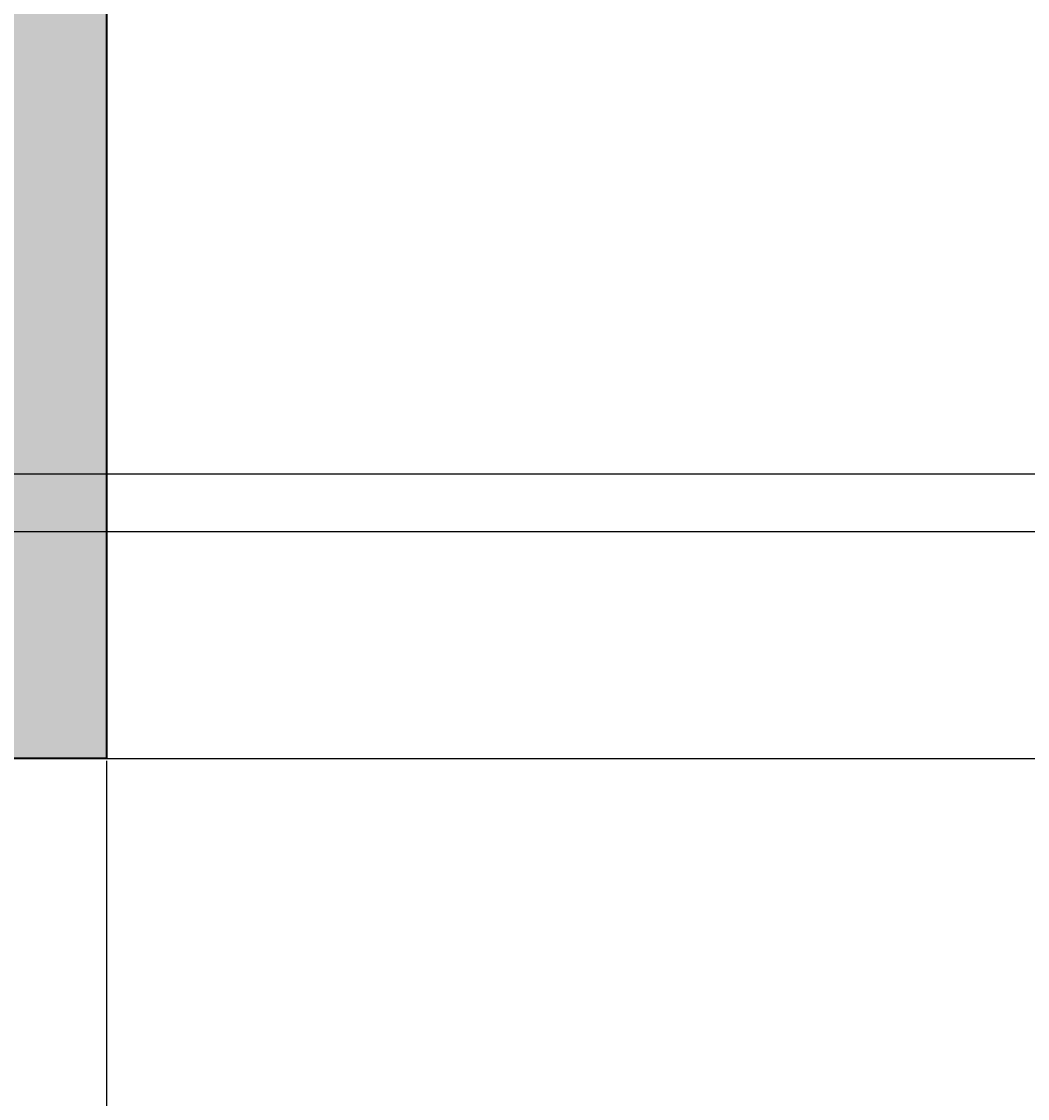
# Model space of a CAD drawing. Units: inches. Extents: x 1998 to 2588, y 1139 to 1977.
# Tile 95 of 134: x 2344 to 2370, y 1580 to 1608. Entities that reach past the tile are written whole.
import ezdxf

# ---------------------------------------------------------------- set-up
doc = ezdxf.new("R2010")
doc.units = ezdxf.units.IN
for name, color, linetype, lineweight in [('A-ANNO-DIMS', 2, 'Continuous', 18), ('A-WALL-PATT', 252, 'Continuous', 13), ('WALL', 200, 'Continuous', 35)]:
    doc.layers.add(name, color=color, linetype=linetype, lineweight=lineweight)
doc.styles.get("Standard").update_dxf_attribs({"font": 'arial.ttf'})
doc.dimstyles.get("Standard").update_dxf_attribs({"dimtxt": 0.18, "dimasz": 0.18, "dimexe": 0.18, "dimexo": 0.0625, "dimgap": 0.09, "dimtad": 0, "dimtih": 1, "dimtoh": 1, "dimdec": 4, "dimzin": 0, "dimdsep": 46, "dimtxsty": 'Standard', "dimcen": 0.09, "dimadec": 0, "dimazin": 0, "dimtfac": 1, "dimtdec": 4, "dimtofl": 0, "dimtmove": 0, "dimatfit": 3, "dimfxl": 1, "dimtolj": 1, "dimtzin": 0, "dimarcsym": 0})

# ---------------------------------------------------------------- blocks, each defined once
blk = doc.blocks.new('*D30')
at = {"layer": 'A-ANNO-DIMS', "color": 0, "lineweight": -2, "transparency": 16777216}
for p, q in [((2407.91, 1636.732), (1997.843, 1636.732)), ((1998.023, 1636.552), (1998.023, 1615.913)), ((1998.023, 1594.912), (1998.023, 1615.552)), ((2407.91, 1594.732), (1997.843, 1594.732))]:
    blk.add_line(p, q, dxfattribs=at)
at = {"layer": 'A-ANNO-DIMS', "color": 0, "transparency": 16777216}
for points in [[(1997.993, 1636.552), (1998.053, 1636.552), (1998.023, 1636.732)], [(1997.993, 1594.912), (1998.053, 1594.912), (1998.023, 1594.732)]]:
    blk.add_solid(points, dxfattribs=at)
at = {"layer": 'Defpoints', "color": 0, "transparency": 16777216}
for p in [(1998.023, 1636.732), (2407.973, 1636.732), (2407.973, 1594.732)]:
    blk.add_point(p, dxfattribs=at)
at = {"layer": 'A-ANNO-DIMS', "color": 0, "transparency": 16777216, "insert": (1998.023, 1615.732), "char_height": 0.18, "attachment_point": 5}
blk.add_mtext('\\A1;42', dxfattribs=at)
blk = doc.blocks.new('*D34')
at = {"layer": 'A-ANNO-DIMS', "color": 0, "lineweight": -2, "transparency": 16777216}
for p, q in [((2407.91, 1594.732), (1997.843, 1594.732)), ((1998.023, 1594.552), (1998.023, 1558.913)), ((1998.023, 1522.912), (1998.023, 1558.552)), ((2407.91, 1522.732), (1997.843, 1522.732))]:
    blk.add_line(p, q, dxfattribs=at)
at = {"layer": 'A-ANNO-DIMS', "color": 0, "transparency": 16777216}
for points in [[(1997.993, 1594.552), (1998.053, 1594.552), (1998.023, 1594.732)], [(1997.993, 1522.912), (1998.053, 1522.912), (1998.023, 1522.732)]]:
    blk.add_solid(points, dxfattribs=at)
at = {"layer": 'Defpoints', "color": 0, "transparency": 16777216}
for p in [(1998.023, 1594.732), (2407.973, 1594.732), (2407.973, 1522.732)]:
    blk.add_point(p, dxfattribs=at)
at = {"layer": 'A-ANNO-DIMS', "color": 0, "transparency": 16777216, "insert": (1998.023, 1558.732), "char_height": 0.18, "attachment_point": 5}
blk.add_mtext('\\A1;72', dxfattribs=at)
blk = doc.blocks.new('*D39')
at = {"layer": 'A-ANNO-DIMS', "color": 0, "lineweight": -2, "transparency": 16777216}
for p, q in [((2115.035, 1628.742), (2588.309, 1628.742)), ((2588.129, 1628.562), (2588.129, 1612.685)), ((2588.129, 1596.444), (2588.129, 1612.321)), ((2115.035, 1596.264), (2588.309, 1596.264))]:
    blk.add_line(p, q, dxfattribs=at)
at = {"layer": 'A-ANNO-DIMS', "color": 0, "transparency": 16777216}
for points in [[(2588.099, 1628.562), (2588.159, 1628.562), (2588.129, 1628.742)], [(2588.099, 1596.444), (2588.159, 1596.444), (2588.129, 1596.264)]]:
    blk.add_solid(points, dxfattribs=at)
at = {"layer": 'Defpoints', "color": 0, "transparency": 16777216}
for p in [(2114.973, 1628.742), (2588.129, 1628.742), (2114.973, 1596.264)]:
    blk.add_point(p, dxfattribs=at)
at = {"layer": 'A-ANNO-DIMS', "color": 0, "transparency": 16777216, "insert": (2588.129, 1612.503), "char_height": 0.18, "attachment_point": 5}
blk.add_mtext('\\A1;32.48', dxfattribs=at)
blk = doc.blocks.new('*D42')
at = {"layer": 'A-ANNO-DIMS', "color": 0, "lineweight": -2, "transparency": 16777216}
for p, q in [((2287.535, 1588.732), (2588.309, 1588.732)), ((2588.129, 1588.552), (2588.129, 1555.914)), ((2588.129, 1522.912), (2588.129, 1555.55)), ((2287.535, 1522.732), (2588.309, 1522.732))]:
    blk.add_line(p, q, dxfattribs=at)
at = {"layer": 'A-ANNO-DIMS', "color": 0, "transparency": 16777216}
for points in [[(2588.099, 1588.552), (2588.159, 1588.552), (2588.129, 1588.732)], [(2588.099, 1522.912), (2588.159, 1522.912), (2588.129, 1522.732)]]:
    blk.add_solid(points, dxfattribs=at)
at = {"layer": 'Defpoints', "color": 0, "transparency": 16777216}
for p in [(2287.473, 1588.732), (2588.129, 1588.732), (2287.473, 1522.732)]:
    blk.add_point(p, dxfattribs=at)
at = {"layer": 'A-ANNO-DIMS', "color": 0, "transparency": 16777216, "insert": (2588.129, 1555.732), "char_height": 0.18, "attachment_point": 5}
blk.add_mtext('\\A1;66', dxfattribs=at)
blk = doc.blocks.new('*D43')
at = {"layer": 'A-ANNO-DIMS', "color": 0, "lineweight": -2, "transparency": 16777216}
for p, q in [((2407.973, 1594.67), (2407.973, 1138.602)), ((2345.973, 1588.67), (2345.973, 1138.602)), ((2346.153, 1138.782), (2376.754, 1138.782)), ((2407.793, 1138.782), (2377.191, 1138.782))]:
    blk.add_line(p, q, dxfattribs=at)
at = {"layer": 'A-ANNO-DIMS', "color": 0, "transparency": 16777216}
for points in [[(2346.153, 1138.812), (2346.153, 1138.752), (2345.973, 1138.782)], [(2407.793, 1138.812), (2407.793, 1138.752), (2407.973, 1138.782)]]:
    blk.add_solid(points, dxfattribs=at)
at = {"layer": 'Defpoints', "color": 0, "transparency": 16777216}
for p in [(2407.973, 1594.732), (2345.973, 1588.732), (2407.973, 1138.782)]:
    blk.add_point(p, dxfattribs=at)
at = {"layer": 'A-ANNO-DIMS', "color": 0, "transparency": 16777216, "insert": (2376.973, 1138.782), "char_height": 0.18, "attachment_point": 5}
blk.add_mtext('\\A1;62', dxfattribs=at)

msp = doc.modelspace()

# ---------------------------------------------------------------- hatches: boundary and pattern name
at = {"layer": 'A-WALL-PATT'}
h = msp.add_hatch(color=256, dxfattribs=at)
h.dxf.hatch_style = 1
h.paths.add_polyline_path([(2222.9729, 1888.7324), (2099.4125, 1888.7324), (2099.4125, 1879.7324), (2222.9729, 1879.7324)])
h.paths.add_polyline_path([(2096.9729, 1868.3278), (2087.9729, 1868.3278), (2087.9729, 1775.637), (2096.9729, 1775.637)])
h.paths.add_polyline_path([(2227.4729, 1868.3278), (2222.9729, 1868.3278), (2222.9729, 1774.3318), (2227.4729, 1774.3318)])
h.paths.add_polyline_path([(2188.3019, 1759.7324), (2138.6074, 1759.7324), (2099.4125, 1759.7324), (2099.4125, 1755.2324), (2176.9729, 1755.2324), (2188.3019, 1755.2324)])
h.paths.add_polyline_path([(2087.9729, 1759.7324), (2059.4729, 1759.7324), (2059.4729, 1702.7324), (2087.9729, 1702.7324), (2087.9729, 1707.2324), (2063.9729, 1707.2324), (2063.9729, 1755.2324), (2087.9729, 1755.2324)])
h.paths.add_polyline_path([(2096.9729, 1755.2324), (2087.9729, 1755.2324), (2087.9729, 1707.2324), (2096.9729, 1707.2324)])
h.paths.add_polyline_path([(2187.0461, 1707.2324), (2105.9729, 1707.2324), (2096.9729, 1707.2324), (2087.9729, 1707.2324), (2087.9729, 1702.7324), (2105.9729, 1702.7324), (2114.9729, 1702.7324), (2187.0461, 1702.7324)])
h.paths.add_polyline_path([(2181.4729, 1719.2028), (2176.9729, 1719.2028), (2176.9729, 1707.2324), (2181.4729, 1707.2324)])
h.paths.add_polyline_path([(2216.0332, 1588.7324), (2114.9729, 1588.7324), (2105.9729, 1588.7324), (2105.9729, 1584.2324), (2216.0332, 1584.2324)])
h.paths.add_polyline_path([(2077.691, 1588.7324), (2061.4729, 1588.7324), (2061.4729, 1584.2324), (2077.691, 1584.2324)])
h.paths.add_polyline_path([(2105.9729, 1588.7324), (2098.0956, 1588.7324), (2098.0956, 1584.2324), (2105.9729, 1584.2324)])
h.paths.add_polyline_path([(2114.9729, 1596.2642), (2110.1012, 1596.2642), (2105.9729, 1596.2642), (2105.9729, 1588.7324), (2114.9729, 1588.7324)])
h.paths.add_polyline_path([(2114.9729, 1584.2324), (2105.9729, 1584.2324), (2105.9729, 1580.249), (2110.1012, 1580.249), (2114.9729, 1580.249)])
h.paths.add_polyline_path([(2114.9729, 1547.7716), (2110.1012, 1547.7716, -0.0318759), (2105.9729, 1548.035), (2105.9729, 1470.2324), (2108.3775, 1470.2324), (2108.3775, 1465.7324), (2186.2943, 1465.7324), (2186.2943, 1470.2324), (2114.9729, 1470.2324)])
h.paths.add_polyline_path([(2227.4729, 1584.2324), (2222.9729, 1584.2324), (2222.9729, 1486.137), (2227.4729, 1486.137)])
h.paths.add_polyline_path([(2295.4138, 1593.2324), (2227.4729, 1593.2324), (2227.4729, 1588.7324), (2295.4138, 1588.7324), (2295.4138, 1591.8729)])
h.paths.add_polyline_path([(2345.9729, 1627.1165), (2341.4729, 1627.1165), (2341.4729, 1593.2324), (2337.2869, 1593.2324), (2337.2869, 1591.8729), (2337.2869, 1588.7324), (2345.9729, 1588.7324)])
h.paths.add_polyline_path([(2291.9729, 1588.7324), (2287.4729, 1588.7324), (2287.4729, 1522.7324), (2291.9729, 1522.7324)])
h.paths.add_polyline_path([(2291.9729, 1522.7324), (2287.4729, 1522.7324), (2227.4729, 1522.7324), (2227.4729, 1518.2324), (2291.9729, 1518.2324)])
h.paths.add_polyline_path([(2295.7347, 1519.5919), (2295.7347, 1522.7324), (2291.9729, 1522.7324), (2291.9729, 1518.2324), (2295.7347, 1518.2324)])
h.paths.add_polyline_path([(2345.9729, 1522.7324), (2337.6078, 1522.7324), (2337.6078, 1519.5919), (2337.6078, 1518.2324), (2341.4729, 1518.2324), (2341.4729, 1488.5616), (2345.9729, 1488.5616)])
h.paths.add_polyline_path([(2345.9729, 1468.1569), (2341.4729, 1468.1569), (2341.4729, 1374.2324), (2227.4729, 1374.2324), (2227.4729, 1369.7324), (2345.9729, 1369.7324)])
h.paths.add_polyline_path([(2345.9729, 1369.7324), (2341.4729, 1369.7324), (2341.4729, 1362.2324), (2345.9729, 1362.2324)])
h.paths.add_polyline_path([(2345.9729, 1317.7324), (2345.9729, 1322.2324), (2341.4729, 1322.2324), (2341.4729, 1285.137), (2345.9729, 1285.137)], flags=17)
h.paths.add_polyline_path([(2356.2096, 1322.2324), (2345.9729, 1322.2324), (2345.9729, 1317.7324), (2356.2096, 1317.7324), (2356.2096, 1319.3088)], flags=17)
h.paths.add_polyline_path([(2393.9729, 1322.2324), (2375.6999, 1322.2324), (2375.6999, 1319.3088, -0.0202458), (2375.636, 1317.7324), (2393.9729, 1317.7324)], flags=17)
h.paths.add_polyline_path([(2398.4729, 1322.2324), (2393.9729, 1322.2324), (2393.9729, 1317.7324), (2393.9729, 1237.7324), (2345.9729, 1237.7324), (2345.9729, 1264.7324), (2341.4729, 1264.7324), (2341.4729, 1228.7324), (2393.9729, 1228.7324), (2482.7412, 1228.7324), (2482.7412, 1237.7324), (2398.4729, 1237.7324), (2398.4729, 1297.1029)])
h.paths.add_polyline_path([(2398.4729, 1362.2324), (2393.9729, 1362.2324), (2393.9729, 1357.7324), (2398.4729, 1357.7324)])
h.paths.add_polyline_path([(2345.9729, 1329.7549), (2341.4729, 1329.7549), (2341.4729, 1322.2324), (2345.9729, 1322.2324)])

# ---------------------------------------------------------------- linework, layer by layer
at = {"layer": 'WALL'}
for p, q in [((2345.9729, 1755.2324), (2345.9729, 1588.7324)), ((2345.9729, 1636.7324), (2345.9729, 1588.7324)), ((2345.9729, 1588.7324), (2337.2869, 1588.7324))]:
    msp.add_line(p, q, dxfattribs=at)

# ---------------------------------------------------------------- dimensions: what is measured, and where the dimension line sits
at = {"layer": 'A-ANNO-DIMS'}
for base, p1, p2, override, picture, middle in [((1998.0229, 1636.7324), (2407.9729, 1594.7324), (2407.9729, 1636.7324), {"dimdec": 0, "dimlfac": 1, "dimrnd": 0, "dimzin": 0, "dimdsep": 46, "dimlunit": 2}, '*D30', (1998.0229, 1615.7324)), ((2588.1286, 1628.7416), (2114.9729, 1596.2642), (2114.9729, 1628.7416), {"dimdec": 2, "dimlfac": 1, "dimrnd": 0, "dimzin": 0, "dimdsep": 46, "dimlunit": 2}, '*D39', (2588.1286, 1612.5029)), ((1998.0229, 1594.7324), (2407.9729, 1522.7324), (2407.9729, 1594.7324), {"dimdec": 0, "dimlfac": 1, "dimrnd": 0, "dimzin": 0, "dimdsep": 46, "dimlunit": 2}, '*D34', (1998.0229, 1558.7324)), ((2588.1286, 1588.7324), (2287.4729, 1522.7324), (2287.4729, 1588.7324), {"dimdec": 0, "dimlfac": 1, "dimrnd": 0, "dimzin": 0, "dimdsep": 46, "dimlunit": 2}, '*D42', (2588.1286, 1555.7324))]:
    dim = msp.add_linear_dim(base=base, p1=p1, p2=p2, angle=90, dimstyle='Standard', override=override, dxfattribs=at)
    dim.commit()
    dim.dimension.update_dxf_attribs({"geometry": picture, "text_midpoint": middle})
dim = msp.add_linear_dim(base=(2407.9729, 1138.7824), p1=(2345.9729, 1588.7324), p2=(2407.9729, 1594.7324), dimstyle='Standard', override={"dimdec": 0, "dimlfac": 1, "dimrnd": 0, "dimzin": 0, "dimdsep": 46, "dimlunit": 2}, dxfattribs=at)
dim.commit()
dim.dimension.update_dxf_attribs({"geometry": '*D43', "text_midpoint": (2376.9729, 1138.7824)})

doc.saveas('drawing.dxf')
